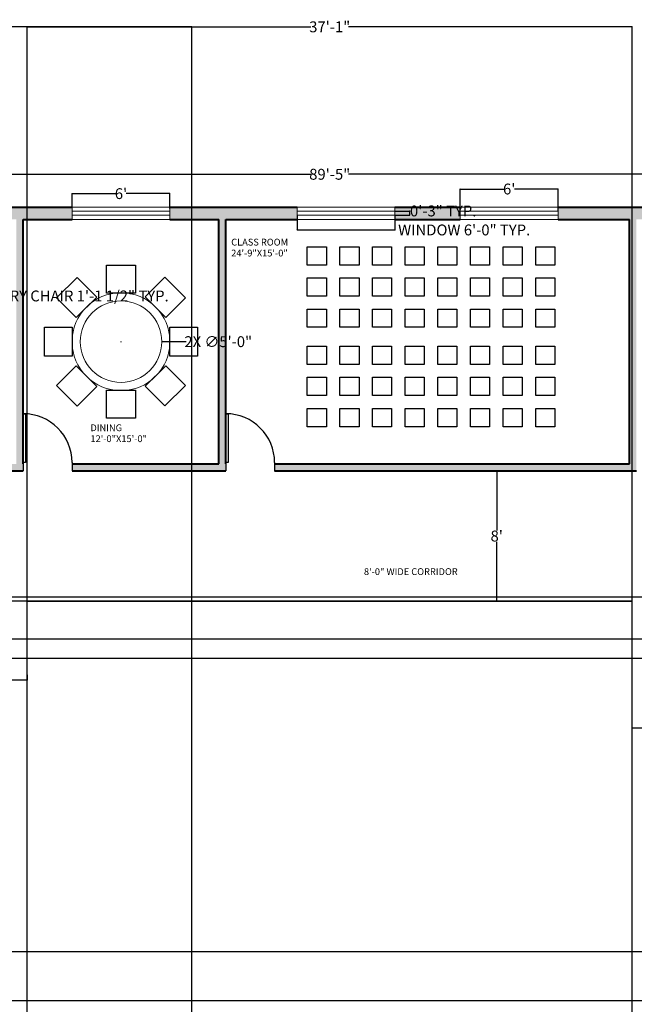
# Model space of a CAD drawing. Units: inches. Extents: x -405 to 940, y 226 to 2032.
# Tile 8 of 10: x 51 to 503, y 1301 to 2026. Entities that reach past the tile are written whole.
import ezdxf

# ---------------------------------------------------------------- set-up
doc = ezdxf.new("R2010")
doc.units = ezdxf.units.IN
doc.header["$MEASUREMENT"] = 0
doc.linetypes.add('ACAD_ISO02W100', pattern=[15, 12, -3])
for name, color, linetype, lineweight in [('A-ANNO-DIMS', 120, 'Continuous', 18), ('A-AREA-IDEN', 32, 'Continuous', 18), ('A-FLOR-EDGE', 3, 'Continuous', 25), ('A-FURN-SEAT', 5, 'Continuous', 18), ('A-GLAZ-HIDN', 1, 'ACAD_ISO02W100', 18), ('A-WALL-PATT', 8, 'Continuous', 13), ('door', 6, 'Continuous', 25), ('tables', 2, 'Continuous', 18), ('wall', 3, 'Continuous', 40), ('window', 1, 'Continuous', 18)]:
    doc.layers.add(name, color=color, linetype=linetype, lineweight=lineweight)
doc.layers.add('beches', color=5, linetype='Continuous')
doc.styles.get("Standard").update_dxf_attribs({"font": 'arial.ttf'})
doc.dimstyles.get("Standard").update_dxf_attribs({"dimtxt": 8, "dimasz": 0.18, "dimexe": 0.18, "dimexo": 0.0625, "dimgap": 0.09, "dimtad": 0, "dimtih": 1, "dimtoh": 1, "dimdec": 0, "dimzin": 0, "dimdsep": 46, "dimlunit": 3, "dimtxsty": 'Standard', "dimblk": 'OBLIQUE', "dimcen": 0.09, "dimadec": 0, "dimazin": 0, "dimtfac": 1, "dimtdec": 0, "dimtofl": 0, "dimtmove": 0, "dimatfit": 3, "dimfxl": 1, "dimtolj": 1, "dimtzin": 0, "dimarcsym": 0})

# ---------------------------------------------------------------- blocks, each defined once
blk = doc.blocks.new('*U4')
for p, q in [((0, 0), (0, -6)), ((36, 0), (36, -6))]:
    blk.add_line(p, q)
blk.add_lwpolyline([(0, 0), (0, 36), (1.75, 36), (1.75, 0)], close=True)
blk.add_arc((0, 0), 36, 0, 90)
blk = doc.blocks.new('*U33')
at = {"layer": 'beches'}
blk.add_lwpolyline([(6.71, -7.02), (-6.71, -7.02), (-6.71, 7.02), (6.71, 7.02)], close=True, dxfattribs=at)
blk = doc.blocks.new('*U34')
at = {"layer": 'A-FURN-SEAT', "transparency": 16777216}
for p in [(-45.84, 168), (-45.84, 168, 12), (-45.84, 168, 24), (-45.84, 168, 36), (-45.84, 168, 48), (-45.84, 168, 60), (-45.84, 168, 72), (-45.84, 168, 84), (-45.84, 168, 96), (-45.84, 168, 108), (-45.84, 168, 120), (-45.84, 168, 132), (-22.92, 168), (-22.92, 168, 12), (-22.92, 168, 24), (-22.92, 168, 36), (-22.92, 168, 48), (-22.92, 168, 60), (-22.92, 168, 72), (-22.92, 168, 84), (-22.92, 168, 96), (-22.92, 168, 108), (-22.92, 168, 120), (-22.92, 168, 132), (0, 168), (0, 168, 12), (0, 168, 24), (0, 168, 36), (0, 168, 48), (0, 168, 60), (0, 168, 72), (0, 168, 84), (0, 168, 96), (0, 168, 108), (0, 168, 120), (0, 168, 132), (-45.84, 144), (-45.84, 144, 12), (-45.84, 144, 24), (-45.84, 144, 36), (-45.84, 144, 48), (-45.84, 144, 60), (-45.84, 144, 72), (-45.84, 144, 84), (-45.84, 144, 96), (-45.84, 144, 108), (-45.84, 144, 120), (-45.84, 144, 132), (-22.92, 144), (-22.92, 144, 12), (-22.92, 144, 24), (-22.92, 144, 36), (-22.92, 144, 48), (-22.92, 144, 60), (-22.92, 144, 72), (-22.92, 144, 84), (-22.92, 144, 96), (-22.92, 144, 108), (-22.92, 144, 120), (-22.92, 144, 132), (0, 144), (0, 144, 12), (0, 144, 24), (0, 144, 36), (0, 144, 48), (0, 144, 60), (0, 144, 72), (0, 144, 84), (0, 144, 96), (0, 144, 108), (0, 144, 120), (0, 144, 132), (-45.84, 120), (-45.84, 120, 12), (-45.84, 120, 24), (-45.84, 120, 36), (-45.84, 120, 48), (-45.84, 120, 60), (-45.84, 120, 72), (-45.84, 120, 84), (-45.84, 120, 96), (-45.84, 120, 108), (-45.84, 120, 120), (-45.84, 120, 132), (-22.92, 120), (-22.92, 120, 12), (-22.92, 120, 24), (-22.92, 120, 36), (-22.92, 120, 48), (-22.92, 120, 60), (-22.92, 120, 72), (-22.92, 120, 84), (-22.92, 120, 96), (-22.92, 120, 108), (-22.92, 120, 120), (-22.92, 120, 132), (0, 120), (0, 120, 12), (0, 120, 24), (0, 120, 36), (0, 120, 48), (0, 120, 60), (0, 120, 72), (0, 120, 84), (0, 120, 96), (0, 120, 108), (0, 120, 120), (0, 120, 132), (-45.84, 96), (-45.84, 96, 12), (-45.84, 96, 24), (-45.84, 96, 36), (-45.84, 96, 48), (-45.84, 96, 60), (-45.84, 96, 72), (-45.84, 96, 84), (-45.84, 96, 96), (-45.84, 96, 108), (-45.84, 96, 120), (-45.84, 96, 132), (-22.92, 96), (-22.92, 96, 12), (-22.92, 96, 24), (-22.92, 96, 36), (-22.92, 96, 48), (-22.92, 96, 60), (-22.92, 96, 72), (-22.92, 96, 84), (-22.92, 96, 96), (-22.92, 96, 108), (-22.92, 96, 120), (-22.92, 96, 132), (0, 96), (0, 96, 12), (0, 96, 24), (0, 96, 36), (0, 96, 48), (0, 96, 60), (0, 96, 72), (0, 96, 84), (0, 96, 96), (0, 96, 108), (0, 96, 120), (0, 96, 132), (-45.84, 72), (-45.84, 72, 12), (-45.84, 72, 24), (-45.84, 72, 36), (-45.84, 72, 48), (-45.84, 72, 60), (-45.84, 72, 72), (-45.84, 72, 84), (-45.84, 72, 96), (-45.84, 72, 108), (-45.84, 72, 120), (-45.84, 72, 132), (-22.92, 72), (-22.92, 72, 12), (-22.92, 72, 24), (-22.92, 72, 36), (-22.92, 72, 48), (-22.92, 72, 60), (-22.92, 72, 72), (-22.92, 72, 84), (-22.92, 72, 96), (-22.92, 72, 108), (-22.92, 72, 120), (-22.92, 72, 132), (0, 72), (0, 72, 12), (0, 72, 24), (0, 72, 36), (0, 72, 48), (0, 72, 60), (0, 72, 72), (0, 72, 84), (0, 72, 96), (0, 72, 108), (0, 72, 120), (0, 72, 132), (-45.84, 48), (-45.84, 48, 12), (-45.84, 48, 24), (-45.84, 48, 36), (-45.84, 48, 48), (-45.84, 48, 60), (-45.84, 48, 72), (-45.84, 48, 84), (-45.84, 48, 96), (-45.84, 48, 108), (-45.84, 48, 120), (-45.84, 48, 132), (-22.92, 48), (-22.92, 48, 12), (-22.92, 48, 24), (-22.92, 48, 36), (-22.92, 48, 48), (-22.92, 48, 60), (-22.92, 48, 72), (-22.92, 48, 84), (-22.92, 48, 96), (-22.92, 48, 108), (-22.92, 48, 120), (-22.92, 48, 132), (0, 48), (0, 48, 12), (0, 48, 24), (0, 48, 36), (0, 48, 48), (0, 48, 60), (0, 48, 72), (0, 48, 84), (0, 48, 96), (0, 48, 108), (0, 48, 120), (0, 48, 132), (-45.84, 24), (-45.84, 24, 12), (-45.84, 24, 24), (-45.84, 24, 36), (-45.84, 24, 48), (-45.84, 24, 60), (-45.84, 24, 72), (-45.84, 24, 84), (-45.84, 24, 96), (-45.84, 24, 108), (-45.84, 24, 120), (-45.84, 24, 132), (-22.92, 24), (-22.92, 24, 12), (-22.92, 24, 24), (-22.92, 24, 36), (-22.92, 24, 48), (-22.92, 24, 60), (-22.92, 24, 72), (-22.92, 24, 84), (-22.92, 24, 96), (-22.92, 24, 108), (-22.92, 24, 120), (-22.92, 24, 132), (0, 24), (0, 24, 12), (0, 24, 24), (0, 24, 36), (0, 24, 48), (0, 24, 60), (0, 24, 72), (0, 24, 84), (0, 24, 96), (0, 24, 108), (0, 24, 120), (0, 24, 132), (-45.84, 0), (-45.84, 0, 12), (-45.84, 0, 24), (-45.84, 0, 36), (-45.84, 0, 48), (-45.84, 0, 60), (-45.84, 0, 72), (-45.84, 0, 84), (-45.84, 0, 96), (-45.84, 0, 108), (-45.84, 0, 120), (-45.84, 0, 132), (-22.92, 0), (-22.92, 0, 12), (-22.92, 0, 24), (-22.92, 0, 36), (-22.92, 0, 48), (-22.92, 0, 60), (-22.92, 0, 72), (-22.92, 0, 84), (-22.92, 0, 96), (-22.92, 0, 108), (-22.92, 0, 120), (-22.92, 0, 132), (0, 0), (0, 0, 12), (0, 0, 24), (0, 0, 36), (0, 0, 48), (0, 0, 60), (0, 0, 72), (0, 0, 84), (0, 0, 96), (0, 0, 108), (0, 0, 120), (0, 0, 132)]:
    blk.add_blockref('*U33', p, dxfattribs=at)
blk = doc.blocks.new('*U31')
at = {"layer": 'beches'}
blk.add_lwpolyline([(6.71, -7.02), (-6.71, -7.02), (-6.71, 7.02), (6.71, 7.02)], close=True, dxfattribs=at)
blk = doc.blocks.new('*U32')
at = {"layer": 'A-FURN-SEAT', "transparency": 16777216}
for p in [(-45.84, 168), (-45.84, 168, 12), (-45.84, 168, 24), (-45.84, 168, 36), (-45.84, 168, 48), (-45.84, 168, 60), (-45.84, 168, 72), (-45.84, 168, 84), (-45.84, 168, 96), (-45.84, 168, 108), (-45.84, 168, 120), (-45.84, 168, 132), (-22.92, 168), (-22.92, 168, 12), (-22.92, 168, 24), (-22.92, 168, 36), (-22.92, 168, 48), (-22.92, 168, 60), (-22.92, 168, 72), (-22.92, 168, 84), (-22.92, 168, 96), (-22.92, 168, 108), (-22.92, 168, 120), (-22.92, 168, 132), (0, 168), (0, 168, 12), (0, 168, 24), (0, 168, 36), (0, 168, 48), (0, 168, 60), (0, 168, 72), (0, 168, 84), (0, 168, 96), (0, 168, 108), (0, 168, 120), (0, 168, 132), (-45.84, 144), (-45.84, 144, 12), (-45.84, 144, 24), (-45.84, 144, 36), (-45.84, 144, 48), (-45.84, 144, 60), (-45.84, 144, 72), (-45.84, 144, 84), (-45.84, 144, 96), (-45.84, 144, 108), (-45.84, 144, 120), (-45.84, 144, 132), (-22.92, 144), (-22.92, 144, 12), (-22.92, 144, 24), (-22.92, 144, 36), (-22.92, 144, 48), (-22.92, 144, 60), (-22.92, 144, 72), (-22.92, 144, 84), (-22.92, 144, 96), (-22.92, 144, 108), (-22.92, 144, 120), (-22.92, 144, 132), (0, 144), (0, 144, 12), (0, 144, 24), (0, 144, 36), (0, 144, 48), (0, 144, 60), (0, 144, 72), (0, 144, 84), (0, 144, 96), (0, 144, 108), (0, 144, 120), (0, 144, 132), (-45.84, 120), (-45.84, 120, 12), (-45.84, 120, 24), (-45.84, 120, 36), (-45.84, 120, 48), (-45.84, 120, 60), (-45.84, 120, 72), (-45.84, 120, 84), (-45.84, 120, 96), (-45.84, 120, 108), (-45.84, 120, 120), (-45.84, 120, 132), (-22.92, 120), (-22.92, 120, 12), (-22.92, 120, 24), (-22.92, 120, 36), (-22.92, 120, 48), (-22.92, 120, 60), (-22.92, 120, 72), (-22.92, 120, 84), (-22.92, 120, 96), (-22.92, 120, 108), (-22.92, 120, 120), (-22.92, 120, 132), (0, 120), (0, 120, 12), (0, 120, 24), (0, 120, 36), (0, 120, 48), (0, 120, 60), (0, 120, 72), (0, 120, 84), (0, 120, 96), (0, 120, 108), (0, 120, 120), (0, 120, 132), (-45.84, 96), (-45.84, 96, 12), (-45.84, 96, 24), (-45.84, 96, 36), (-45.84, 96, 48), (-45.84, 96, 60), (-45.84, 96, 72), (-45.84, 96, 84), (-45.84, 96, 96), (-45.84, 96, 108), (-45.84, 96, 120), (-45.84, 96, 132), (-22.92, 96), (-22.92, 96, 12), (-22.92, 96, 24), (-22.92, 96, 36), (-22.92, 96, 48), (-22.92, 96, 60), (-22.92, 96, 72), (-22.92, 96, 84), (-22.92, 96, 96), (-22.92, 96, 108), (-22.92, 96, 120), (-22.92, 96, 132), (0, 96), (0, 96, 12), (0, 96, 24), (0, 96, 36), (0, 96, 48), (0, 96, 60), (0, 96, 72), (0, 96, 84), (0, 96, 96), (0, 96, 108), (0, 96, 120), (0, 96, 132), (-45.84, 72), (-45.84, 72, 12), (-45.84, 72, 24), (-45.84, 72, 36), (-45.84, 72, 48), (-45.84, 72, 60), (-45.84, 72, 72), (-45.84, 72, 84), (-45.84, 72, 96), (-45.84, 72, 108), (-45.84, 72, 120), (-45.84, 72, 132), (-22.92, 72), (-22.92, 72, 12), (-22.92, 72, 24), (-22.92, 72, 36), (-22.92, 72, 48), (-22.92, 72, 60), (-22.92, 72, 72), (-22.92, 72, 84), (-22.92, 72, 96), (-22.92, 72, 108), (-22.92, 72, 120), (-22.92, 72, 132), (0, 72), (0, 72, 12), (0, 72, 24), (0, 72, 36), (0, 72, 48), (0, 72, 60), (0, 72, 72), (0, 72, 84), (0, 72, 96), (0, 72, 108), (0, 72, 120), (0, 72, 132), (-45.84, 48), (-45.84, 48, 12), (-45.84, 48, 24), (-45.84, 48, 36), (-45.84, 48, 48), (-45.84, 48, 60), (-45.84, 48, 72), (-45.84, 48, 84), (-45.84, 48, 96), (-45.84, 48, 108), (-45.84, 48, 120), (-45.84, 48, 132), (-22.92, 48), (-22.92, 48, 12), (-22.92, 48, 24), (-22.92, 48, 36), (-22.92, 48, 48), (-22.92, 48, 60), (-22.92, 48, 72), (-22.92, 48, 84), (-22.92, 48, 96), (-22.92, 48, 108), (-22.92, 48, 120), (-22.92, 48, 132), (0, 48), (0, 48, 12), (0, 48, 24), (0, 48, 36), (0, 48, 48), (0, 48, 60), (0, 48, 72), (0, 48, 84), (0, 48, 96), (0, 48, 108), (0, 48, 120), (0, 48, 132), (-45.84, 24), (-45.84, 24, 12), (-45.84, 24, 24), (-45.84, 24, 36), (-45.84, 24, 48), (-45.84, 24, 60), (-45.84, 24, 72), (-45.84, 24, 84), (-45.84, 24, 96), (-45.84, 24, 108), (-45.84, 24, 120), (-45.84, 24, 132), (-22.92, 24), (-22.92, 24, 12), (-22.92, 24, 24), (-22.92, 24, 36), (-22.92, 24, 48), (-22.92, 24, 60), (-22.92, 24, 72), (-22.92, 24, 84), (-22.92, 24, 96), (-22.92, 24, 108), (-22.92, 24, 120), (-22.92, 24, 132), (0, 24), (0, 24, 12), (0, 24, 24), (0, 24, 36), (0, 24, 48), (0, 24, 60), (0, 24, 72), (0, 24, 84), (0, 24, 96), (0, 24, 108), (0, 24, 120), (0, 24, 132), (-45.84, 0), (-45.84, 0, 12), (-45.84, 0, 24), (-45.84, 0, 36), (-45.84, 0, 48), (-45.84, 0, 60), (-45.84, 0, 72), (-45.84, 0, 84), (-45.84, 0, 96), (-45.84, 0, 108), (-45.84, 0, 120), (-45.84, 0, 132), (-22.92, 0), (-22.92, 0, 12), (-22.92, 0, 24), (-22.92, 0, 36), (-22.92, 0, 48), (-22.92, 0, 60), (-22.92, 0, 72), (-22.92, 0, 84), (-22.92, 0, 96), (-22.92, 0, 108), (-22.92, 0, 120), (-22.92, 0, 132), (0, 0), (0, 0, 12), (0, 0, 24), (0, 0, 36), (0, 0, 48), (0, 0, 60), (0, 0, 72), (0, 0, 84), (0, 0, 96), (0, 0, 108), (0, 0, 120), (0, 0, 132)]:
    blk.add_blockref('*U31', p, dxfattribs=at)
blk = doc.blocks.new('*U35')
at = {"layer": 'beches'}
blk.add_lwpolyline([(-10.7, 10.22), (10.7, 10.22), (10.7, -10.22), (-10.7, -10.22)], close=True, dxfattribs=at)
blk = doc.blocks.new('*U36')
at = {"layer": 'A-FURN-SEAT', "transparency": 16777216}
blk.add_blockref('*U35', (125.75, 1834.83), dxfattribs=at)
for p, rotation in [((93.21, 1821.33), 45.00000000000002), ((158.29, 1821.37), 314.9999999999999), ((79.75, 1788.79), 90.00000000000003), ((171.79, 1788.83), 270), ((93.24, 1756.26), 135), ((158.32, 1756.29), 225), ((125.79, 1742.79), 180)]:
    blk.add_blockref('*U35', p, dxfattribs=dict(at, rotation=rotation))
blk = doc.blocks.new('_Oblique')
at = {"color": 0, "linetype": 'ByBlock', "lineweight": -2}
blk.add_line((-0.5, -0.5), (0.5, 0.5), dxfattribs=at)
blk = doc.blocks.new('*D40')
at = {"layer": 'A-ANNO-DIMS', "color": 0, "lineweight": -2, "transparency": 16777216}
for p, q in [((-39.23, 1543.59), (-39.23, 1539.64)), ((56.77, 1543.59), (56.77, 1539.64)), ((-39.23, 1539.82), (4.99, 1539.82)), ((56.77, 1539.82), (12.54, 1539.82))]:
    blk.add_line(p, q, dxfattribs=at)
at = {"layer": 'Defpoints', "color": 0, "transparency": 16777216}
for p in [(-39.23, 1543.65), (56.77, 1543.65), (56.77, 1539.82)]:
    blk.add_point(p, dxfattribs=at)
at = {"layer": 'A-ANNO-DIMS', "color": 0, "lineweight": -2, "transparency": 16777216, "xscale": 0.18, "yscale": 0.18, "zscale": 0.18, "rotation": 180}
blk.add_blockref('_Oblique', (-39.23, 1539.82), dxfattribs=at)
at = {"layer": 'A-ANNO-DIMS', "color": 0, "lineweight": -2, "transparency": 16777216, "xscale": 0.18, "yscale": 0.18, "zscale": 0.18}
blk.add_blockref('_Oblique', (56.77, 1539.82), dxfattribs=at)
at = {"layer": 'A-ANNO-DIMS', "color": 0, "transparency": 16777216, "insert": (8.77, 1539.82), "char_height": 8, "attachment_point": 5}
blk.add_mtext("\\A1;8'", dxfattribs=at)
blk = doc.blocks.new('*D41')
at = {"layer": 'A-ANNO-DIMS', "color": 0, "lineweight": -2, "transparency": 16777216}
for p, q in [((405.58, 1693.81), (401.92, 1693.81)), ((402.1, 1693.81), (402.1, 1649.98)), ((402.1, 1597.81), (402.1, 1641.64)), ((405.58, 1597.81), (401.92, 1597.81))]:
    blk.add_line(p, q, dxfattribs=at)
at = {"layer": 'Defpoints', "color": 0, "transparency": 16777216}
for p in [(405.64, 1693.81), (402.1, 1597.81), (405.64, 1597.81)]:
    blk.add_point(p, dxfattribs=at)
at = {"layer": 'A-ANNO-DIMS', "color": 0, "lineweight": -2, "transparency": 16777216, "xscale": 0.18, "yscale": 0.18, "zscale": 0.18}
for p, rotation in [((402.1, 1693.81), 90), ((402.1, 1597.81), 270)]:
    blk.add_blockref('_Oblique', p, dxfattribs=dict(at, rotation=rotation))
at = {"layer": 'A-ANNO-DIMS', "color": 0, "transparency": 16777216, "insert": (402.1, 1645.81), "char_height": 8, "attachment_point": 5}
blk.add_mtext("\\A1;8'", dxfattribs=at)
blk = doc.blocks.new('*D42')
at = {"layer": 'A-ANNO-DIMS', "color": 0, "lineweight": -2, "transparency": 16777216}
for p, q in [((501.77, 1498.93), (501.77, 1504.9)), ((501.77, 1504.72), (545.99, 1504.72)), ((597.77, 1504.72), (553.54, 1504.72)), ((597.77, 1498.93), (597.77, 1504.9))]:
    blk.add_line(p, q, dxfattribs=at)
at = {"layer": 'Defpoints', "color": 0, "transparency": 16777216}
for p in [(501.77, 1504.72), (501.77, 1498.87), (597.77, 1498.87)]:
    blk.add_point(p, dxfattribs=at)
at = {"layer": 'A-ANNO-DIMS', "color": 0, "lineweight": -2, "transparency": 16777216, "xscale": 0.18, "yscale": 0.18, "zscale": 0.18, "rotation": 180}
blk.add_blockref('_Oblique', (501.77, 1504.72), dxfattribs=at)
at = {"layer": 'A-ANNO-DIMS', "color": 0, "lineweight": -2, "transparency": 16777216, "xscale": 0.18, "yscale": 0.18, "zscale": 0.18}
blk.add_blockref('_Oblique', (597.77, 1504.72), dxfattribs=at)
at = {"layer": 'A-ANNO-DIMS', "color": 0, "transparency": 16777216, "insert": (549.77, 1504.72), "char_height": 8, "attachment_point": 5}
blk.add_mtext("\\A1;8'", dxfattribs=at)
blk = doc.blocks.new('*D43')
at = {"layer": 'A-ANNO-DIMS', "color": 0, "lineweight": -2, "transparency": 16777216}
for p, q in [((-257.23, 1887.87), (-257.23, 1912.15)), ((-257.23, 1911.97), (265.43, 1911.97)), ((815.77, 1911.97), (293.1, 1911.97)), ((815.77, 1887.87), (815.77, 1912.15))]:
    blk.add_line(p, q, dxfattribs=at)
at = {"layer": 'Defpoints', "color": 0, "transparency": 16777216}
for p in [(815.77, 1911.97), (-257.23, 1887.81), (815.77, 1887.81)]:
    blk.add_point(p, dxfattribs=at)
at = {"layer": 'A-ANNO-DIMS', "color": 0, "lineweight": -2, "transparency": 16777216, "xscale": 0.18, "yscale": 0.18, "zscale": 0.18, "rotation": 180}
blk.add_blockref('_Oblique', (-257.23, 1911.97), dxfattribs=at)
at = {"layer": 'A-ANNO-DIMS', "color": 0, "lineweight": -2, "transparency": 16777216, "xscale": 0.18, "yscale": 0.18, "zscale": 0.18}
blk.add_blockref('_Oblique', (815.77, 1911.97), dxfattribs=at)
at = {"layer": 'A-ANNO-DIMS', "color": 0, "transparency": 16777216, "insert": (279.27, 1911.97), "char_height": 8, "attachment_point": 5}
blk.add_mtext('\\A1;89\'-5"', dxfattribs=at)
blk = doc.blocks.new('*D63')
at = {"layer": 'A-ANNO-DIMS', "color": 0, "lineweight": -2, "transparency": 16777216}
for p, q in [((89.77, 1887.87), (89.77, 1897.91)), ((89.77, 1897.73), (121.98, 1897.73)), ((161.77, 1897.73), (129.56, 1897.73)), ((161.77, 1886.78), (161.77, 1897.91))]:
    blk.add_line(p, q, dxfattribs=at)
at = {"layer": 'Defpoints', "color": 0, "transparency": 16777216}
for p in [(161.77, 1897.73), (89.77, 1887.81), (161.77, 1886.72)]:
    blk.add_point(p, dxfattribs=at)
at = {"layer": 'A-ANNO-DIMS', "color": 0, "lineweight": -2, "transparency": 16777216, "xscale": 0.18, "yscale": 0.18, "zscale": 0.18, "rotation": 180}
blk.add_blockref('_Oblique', (89.77, 1897.73), dxfattribs=at)
at = {"layer": 'A-ANNO-DIMS', "color": 0, "lineweight": -2, "transparency": 16777216, "xscale": 0.18, "yscale": 0.18, "zscale": 0.18}
blk.add_blockref('_Oblique', (161.77, 1897.73), dxfattribs=at)
at = {"layer": 'A-ANNO-DIMS', "color": 0, "transparency": 16777216, "insert": (125.77, 1897.73), "char_height": 8, "attachment_point": 5}
blk.add_mtext("\\A1;6'", dxfattribs=at)
blk = doc.blocks.new('*D64')
at = {"layer": 'A-ANNO-DIMS', "color": 0, "lineweight": -2, "transparency": 16777216}
for p, q in [((375.27, 1884.87), (375.27, 1901.31)), ((375.27, 1901.13), (407.48, 1901.13)), ((447.27, 1901.13), (415.06, 1901.13)), ((447.27, 1884.87), (447.27, 1901.31))]:
    blk.add_line(p, q, dxfattribs=at)
at = {"layer": 'Defpoints', "color": 0, "transparency": 16777216}
for p in [(447.27, 1901.13), (375.27, 1884.81), (447.27, 1884.81)]:
    blk.add_point(p, dxfattribs=at)
at = {"layer": 'A-ANNO-DIMS', "color": 0, "lineweight": -2, "transparency": 16777216, "xscale": 0.18, "yscale": 0.18, "zscale": 0.18, "rotation": 180}
blk.add_blockref('_Oblique', (375.27, 1901.13), dxfattribs=at)
at = {"layer": 'A-ANNO-DIMS', "color": 0, "lineweight": -2, "transparency": 16777216, "xscale": 0.18, "yscale": 0.18, "zscale": 0.18}
blk.add_blockref('_Oblique', (447.27, 1901.13), dxfattribs=at)
at = {"layer": 'A-ANNO-DIMS', "color": 0, "transparency": 16777216, "insert": (411.27, 1901.13), "char_height": 8, "attachment_point": 5}
blk.add_mtext("\\A1;6'", dxfattribs=at)
blk = doc.blocks.new('TABLE-ROUND-72IN')
for radius in [36, 30]:
    blk.add_circle((36, 36), radius)
blk = doc.blocks.new('WIN-PANE-72IN')
for p, q in [((0, 3), (72, 3)), ((0, 0), (72, 0))]:
    blk.add_line(p, q)
blk = doc.blocks.new('*D83')
at = {"layer": 'A-ANNO-DIMS', "color": 0, "lineweight": -2, "transparency": 16777216}
for p, q in [((255.27, 1881.75), (255.27, 1870.83)), ((327.27, 1881.75), (327.27, 1870.83)), ((255.27, 1871.01), (327.27, 1871.01)), ((327.27, 1871.01), (327.45, 1871.01))]:
    blk.add_line(p, q, dxfattribs=at)
at = {"layer": 'Defpoints', "color": 0, "transparency": 16777216}
for p in [(255.27, 1881.81), (327.27, 1881.81), (327.27, 1871.01)]:
    blk.add_point(p, dxfattribs=at)
at = {"layer": 'A-ANNO-DIMS', "color": 0, "lineweight": -2, "transparency": 16777216, "xscale": 0.18, "yscale": 0.18, "zscale": 0.18, "rotation": 180}
blk.add_blockref('_Oblique', (255.27, 1871.01), dxfattribs=at)
at = {"layer": 'A-ANNO-DIMS', "color": 0, "lineweight": -2, "transparency": 16777216, "xscale": 0.18, "yscale": 0.18, "zscale": 0.18}
blk.add_blockref('_Oblique', (327.27, 1871.01), dxfattribs=at)
at = {"layer": 'A-ANNO-DIMS', "color": 0, "transparency": 16777216, "insert": (378.16, 1871.01), "char_height": 8, "attachment_point": 5}
blk.add_mtext('\\A1;WINDOW 6\'-0" TYP.', dxfattribs=at)
blk = doc.blocks.new('*D84')
at = {"layer": 'A-ANNO-DIMS', "color": 0, "lineweight": -2, "transparency": 16777216}
for p, q in [((327.33, 1884.81), (338.25, 1884.81)), ((338.07, 1884.81), (338.07, 1884.99)), ((338.07, 1884.99), (338.25, 1884.99)), ((338.07, 1881.81), (338.07, 1884.81)), ((327.33, 1881.81), (338.25, 1881.81))]:
    blk.add_line(p, q, dxfattribs=at)
at = {"layer": 'Defpoints', "color": 0, "transparency": 16777216}
for p in [(327.27, 1884.81), (338.07, 1884.81), (327.27, 1881.81)]:
    blk.add_point(p, dxfattribs=at)
at = {"layer": 'A-ANNO-DIMS', "color": 0, "lineweight": -2, "transparency": 16777216, "xscale": 0.18, "yscale": 0.18, "zscale": 0.18}
for p, rotation in [((338.07, 1884.81), 90), ((338.07, 1881.81), 270)]:
    blk.add_blockref('_Oblique', p, dxfattribs=dict(at, rotation=rotation))
at = {"layer": 'A-ANNO-DIMS', "color": 0, "transparency": 16777216, "insert": (362.72, 1884.99), "char_height": 8, "attachment_point": 5}
blk.add_mtext('\\A1;0\'-3" TYP.', dxfattribs=at)
blk = doc.blocks.new('*D91')
at = {"layer": 'A-ANNO-DIMS', "color": 0, "lineweight": -2, "transparency": 16777216}
for p, q in [((-2.26, 1824.45), (-2.26, 1822.27)), ((-2.26, 1822.45), (11.46, 1822.45)), ((11.46, 1824.45), (11.46, 1822.27)), ((11.46, 1822.45), (11.64, 1822.45))]:
    blk.add_line(p, q, dxfattribs=at)
at = {"layer": 'Defpoints', "color": 0, "transparency": 16777216}
for p in [(-2.26, 1824.51), (11.46, 1824.51), (11.46, 1822.45)]:
    blk.add_point(p, dxfattribs=at)
at = {"layer": 'A-ANNO-DIMS', "color": 0, "lineweight": -2, "transparency": 16777216, "xscale": 0.18, "yscale": 0.18, "zscale": 0.18, "rotation": 180}
blk.add_blockref('_Oblique', (-2.26, 1822.45), dxfattribs=at)
at = {"layer": 'A-ANNO-DIMS', "color": 0, "lineweight": -2, "transparency": 16777216, "xscale": 0.18, "yscale": 0.18, "zscale": 0.18}
blk.add_blockref('_Oblique', (11.46, 1822.45), dxfattribs=at)
at = {"layer": 'A-ANNO-DIMS', "color": 0, "transparency": 16777216, "insert": (88.39, 1822.45), "char_height": 8, "attachment_point": 5}
blk.add_mtext('\\A1;PANTRY CHAIR 1\'-1 1/2" TYP.', dxfattribs=at)
blk = doc.blocks.new('*D100')
at = {"layer": 'A-ANNO-DIMS', "color": 0, "lineweight": -2, "transparency": 16777216}
for p, q in [((626.71, 1569.84), (-390.06, 1569.84)), ((-389.88, 1569.84), (-389.88, 1566.93)), ((-389.88, 1555.81), (-389.88, 1558.72)), ((626.71, 1555.81), (-390.06, 1555.81))]:
    blk.add_line(p, q, dxfattribs=at)
at = {"layer": 'Defpoints', "color": 0, "transparency": 16777216}
for p in [(626.77, 1569.84), (-389.88, 1555.81), (626.77, 1555.81)]:
    blk.add_point(p, dxfattribs=at)
at = {"layer": 'A-ANNO-DIMS', "color": 0, "lineweight": -2, "transparency": 16777216, "xscale": 0.18, "yscale": 0.18, "zscale": 0.18}
for p, rotation in [((-389.88, 1569.84), 90), ((-389.88, 1555.81), 270)]:
    blk.add_blockref('_Oblique', p, dxfattribs=dict(at, rotation=rotation))
at = {"layer": 'A-ANNO-DIMS', "color": 0, "transparency": 16777216, "insert": (-389.88, 1562.83), "char_height": 8, "attachment_point": 5}
blk.add_mtext('\\A1;1\'-2"', dxfattribs=at)
blk = doc.blocks.new('*D105')
at = {"layer": 'A-ANNO-DIMS', "color": 0, "lineweight": -2, "transparency": 16777216}
for p, q in [((602.71, 1600.81), (-390.06, 1600.81)), ((-389.88, 1600.81), (-389.88, 1589.43)), ((-389.88, 1569.84), (-389.88, 1581.22)), ((626.71, 1569.84), (-390.06, 1569.84))]:
    blk.add_line(p, q, dxfattribs=at)
at = {"layer": 'Defpoints', "color": 0, "transparency": 16777216}
for p in [(602.77, 1600.81), (-389.88, 1569.84), (626.77, 1569.84)]:
    blk.add_point(p, dxfattribs=at)
at = {"layer": 'A-ANNO-DIMS', "color": 0, "lineweight": -2, "transparency": 16777216, "xscale": 0.18, "yscale": 0.18, "zscale": 0.18}
for p, rotation in [((-389.88, 1600.81), 90), ((-389.88, 1569.84), 270)]:
    blk.add_blockref('_Oblique', p, dxfattribs=dict(at, rotation=rotation))
at = {"layer": 'A-ANNO-DIMS', "color": 0, "transparency": 16777216, "insert": (-389.88, 1585.33), "char_height": 8, "attachment_point": 5}
blk.add_mtext('\\A1;2\'-7"', dxfattribs=at)
blk = doc.blocks.new('*D106')
at = {"layer": 'A-ANNO-DIMS', "color": 0, "lineweight": -2, "transparency": 16777216}
for p, q in [((56.77, 851.87), (56.77, 2020.64)), ((56.77, 2020.46), (265.44, 2020.46)), ((501.77, 2020.46), (293.1, 2020.46)), ((501.77, 851.87), (501.77, 2020.64))]:
    blk.add_line(p, q, dxfattribs=at)
at = {"layer": 'Defpoints', "color": 0, "transparency": 16777216}
for p in [(501.77, 2020.46), (56.77, 851.81), (501.77, 851.81)]:
    blk.add_point(p, dxfattribs=at)
at = {"layer": 'A-ANNO-DIMS', "color": 0, "lineweight": -2, "transparency": 16777216, "xscale": 0.18, "yscale": 0.18, "zscale": 0.18, "rotation": 180}
blk.add_blockref('_Oblique', (56.77, 2020.46), dxfattribs=at)
at = {"layer": 'A-ANNO-DIMS', "color": 0, "lineweight": -2, "transparency": 16777216, "xscale": 0.18, "yscale": 0.18, "zscale": 0.18}
blk.add_blockref('_Oblique', (501.77, 2020.46), dxfattribs=at)
at = {"layer": 'A-ANNO-DIMS', "color": 0, "transparency": 16777216, "insert": (279.27, 2020.46), "char_height": 8, "attachment_point": 5}
blk.add_mtext('\\A1;37\'-1"', dxfattribs=at)
blk = doc.blocks.new('*D107')
at = {"layer": 'A-ANNO-DIMS', "color": 0, "lineweight": -2, "transparency": 16777216}
for p, q in [((501.71, 1597.81), (-390.06, 1597.81)), ((-389.88, 1597.81), (-389.88, 1228.98)), ((-389.88, 851.81), (-389.88, 1220.64)), ((501.71, 851.81), (-390.06, 851.81))]:
    blk.add_line(p, q, dxfattribs=at)
at = {"layer": 'Defpoints', "color": 0, "transparency": 16777216}
for p in [(-389.88, 1597.81), (501.77, 1597.81), (501.77, 851.81)]:
    blk.add_point(p, dxfattribs=at)
at = {"layer": 'A-ANNO-DIMS', "color": 0, "lineweight": -2, "transparency": 16777216, "xscale": 0.18, "yscale": 0.18, "zscale": 0.18}
for p, rotation in [((-389.88, 1597.81), 90), ((-389.88, 851.81), 270)]:
    blk.add_blockref('_Oblique', p, dxfattribs=dict(at, rotation=rotation))
at = {"layer": 'A-ANNO-DIMS', "color": 0, "transparency": 16777216, "insert": (-389.88, 1224.81), "char_height": 8, "attachment_point": 5}
blk.add_mtext('\\A1;62\'-2"', dxfattribs=at)
blk = doc.blocks.new('*D109')
at = {"layer": 'A-ANNO-DIMS', "color": 0, "lineweight": -2, "transparency": 16777216}
for p, q in [((-248.23, 750.87), (-248.23, 2020.64)), ((-248.23, 2020.46), (-49.06, 2020.46)), ((177.77, 2020.46), (-21.4, 2020.46)), ((177.77, 750.87), (177.77, 2020.64))]:
    blk.add_line(p, q, dxfattribs=at)
at = {"layer": 'Defpoints', "color": 0, "transparency": 16777216}
for p in [(177.77, 2020.46), (-248.23, 750.81), (177.77, 750.81)]:
    blk.add_point(p, dxfattribs=at)
at = {"layer": 'A-ANNO-DIMS', "color": 0, "lineweight": -2, "transparency": 16777216, "xscale": 0.18, "yscale": 0.18, "zscale": 0.18, "rotation": 180}
blk.add_blockref('_Oblique', (-248.23, 2020.46), dxfattribs=at)
at = {"layer": 'A-ANNO-DIMS', "color": 0, "lineweight": -2, "transparency": 16777216, "xscale": 0.18, "yscale": 0.18, "zscale": 0.18}
blk.add_blockref('_Oblique', (177.77, 2020.46), dxfattribs=at)
at = {"layer": 'A-ANNO-DIMS', "color": 0, "transparency": 16777216, "insert": (-35.23, 2020.46), "char_height": 8, "attachment_point": 5}
blk.add_mtext('\\A1;35\'-6"', dxfattribs=at)
blk = doc.blocks.new('*D114')
at = {"layer": 'A-ANNO-DIMS', "color": 0, "lineweight": -2, "transparency": 16777216}
for p, q in [((602.71, 1339.81), (-390.06, 1339.81)), ((-389.88, 1339.81), (-389.88, 1325.99)), ((-389.88, 1303.81), (-389.88, 1317.63)), ((602.71, 1303.81), (-390.06, 1303.81))]:
    blk.add_line(p, q, dxfattribs=at)
at = {"layer": 'Defpoints', "color": 0, "transparency": 16777216}
for p in [(602.77, 1339.81), (-389.88, 1303.81), (602.77, 1303.81)]:
    blk.add_point(p, dxfattribs=at)
at = {"layer": 'A-ANNO-DIMS', "color": 0, "lineweight": -2, "transparency": 16777216, "xscale": 0.18, "yscale": 0.18, "zscale": 0.18}
for p, rotation in [((-389.88, 1339.81), 90), ((-389.88, 1303.81), 270)]:
    blk.add_blockref('_Oblique', p, dxfattribs=dict(at, rotation=rotation))
at = {"layer": 'A-ANNO-DIMS', "color": 0, "transparency": 16777216, "insert": (-389.88, 1321.81), "char_height": 8, "attachment_point": 5}
blk.add_mtext('\\A1;3\'-0"', dxfattribs=at)
blk = doc.blocks.new('*D118')
at = {"layer": 'A-ANNO-DIMS', "color": 0, "lineweight": -2, "transparency": 16777216}
for p, q in [((125.68, 1788.81), (125.86, 1788.81)), ((125.77, 1788.72), (125.77, 1788.9)), ((173.77, 1788.81), (155.77, 1788.81))]:
    blk.add_line(p, q, dxfattribs=at)
at = {"layer": 'Defpoints', "color": 0, "transparency": 16777216}
for p in [(95.77, 1788.81), (155.77, 1788.81)]:
    blk.add_point(p, dxfattribs=at)
at = {"layer": 'A-ANNO-DIMS', "color": 0, "lineweight": -2, "transparency": 16777216, "xscale": 0.18, "yscale": 0.18, "zscale": 0.18, "rotation": 179.9996944225092}
blk.add_blockref('_Oblique', (155.77, 1788.81), dxfattribs=at)
at = {"layer": 'A-ANNO-DIMS', "color": 0, "transparency": 16777216, "insert": (197.29, 1788.81), "char_height": 8, "attachment_point": 5}
blk.add_mtext('\\A1;2X ∅5\'-0"', dxfattribs=at)

msp = doc.modelspace()

# ---------------------------------------------------------------- hatches: boundary and pattern name
at = {"layer": 'A-WALL-PATT'}
h = msp.add_hatch(dxfattribs=at)
h.set_pattern_fill('AR-HBONE', color=256)
h.set_pattern_definition([(45, (599.8442, 904.9158), (0, 5.656854), [12, -4]), (135, (602.6726, 907.744), (4e-16, 5.656854), [12, -4])])
h.paths.add_polyline_path([(-248.23, 1045.81), (-257.23, 1045.81), (-257.23, 964.81), (-248.23, 964.81)], flags=17)
h.paths.add_polyline_path([(-248.23, 851.81), (-39.23, 851.81), (-39.23, 856.81), (-44.23, 856.81), (-248.23, 856.81), (-248.23, 892.81), (-257.23, 892.81), (-257.23, 839.81), (-248.23, 839.81)])
h.paths.add_polyline_path([(-248.23, 750.81), (124.74, 750.81), (124.74, 751.73), (124.74, 755.81), (-248.23, 755.81), (-248.23, 767.81), (-257.23, 767.81), (-257.23, 726.81), (-248.23, 726.81)])
h.paths.add_polyline_path([(-248.23, 654.81), (-257.23, 654.81), (-257.23, 630.81), (-248.23, 630.81)])
h.paths.add_polyline_path([(-180.23, 534.81), (-248.23, 534.81), (-248.23, 558.81), (-257.23, 558.81), (-257.23, 525.81), (-180.23, 525.81)])
h.paths.add_polyline_path([(-69.23, 534.81), (-108.23, 534.81), (-108.23, 525.81), (-69.23, 525.81)])
h.paths.add_polyline_path([(35.77, 534.81), (2.77, 534.81), (2.77, 525.81), (35.77, 525.81)])
h.paths.add_polyline_path([(182.77, 755.81), (160.74, 755.81), (160.74, 750.81), (177.77, 750.81), (177.77, 534.81), (107.77, 534.81), (107.77, 525.81), (182.77, 525.81)])
h.paths.add_polyline_path([(-39.23, 1609.81), (-44.23, 1609.81), (-44.23, 1604.81), (-44.23, 1460.81), (-135.23, 1460.81), (-135.23, 1465.73), (-140.23, 1465.73), (-140.23, 1460.81), (-248.23, 1460.81), (-248.23, 1471.31), (-257.23, 1471.31), (-257.23, 1419.81), (-248.23, 1419.81), (-248.23, 1455.81), (-44.23, 1455.81), (-44.23, 1194.81), (-39.23, 1194.81)])
h.paths.add_polyline_path([(-248.23, 1520.81), (-257.23, 1520.81), (-257.23, 1495.31), (-248.23, 1495.31), (-248.23, 1505.81), (-140.23, 1505.81), (-140.23, 1495.73), (-135.23, 1495.73), (-135.23, 1516.79), (-140.23, 1516.79), (-140.23, 1510.81), (-248.23, 1510.81)], flags=17)
h.paths.add_polyline_path([(-248.23, 1570.31), (-257.23, 1570.31), (-257.23, 1544.81), (-248.23, 1544.81), (-248.23, 1554.81), (-140.23, 1554.81), (-140.23, 1546.79), (-135.23, 1546.79), (-135.23, 1565.08), (-140.23, 1565.08), (-140.23, 1559.81), (-248.23, 1559.81)], flags=17)
h.paths.add_polyline_path([(-248.23, 1615.81), (-257.23, 1615.81), (-257.23, 1594.31), (-248.23, 1594.31), (-248.23, 1604.81), (-140.23, 1604.81), (-140.23, 1595.08), (-135.23, 1595.08), (-135.23, 1604.81), (-80.23, 1604.81), (-80.23, 1609.81), (-248.23, 1609.81)])
h.paths.add_polyline_path([(-248.23, 1783.81), (-235.46, 1783.81), (-235.46, 1788.81), (-248.23, 1788.81), (-248.23, 1878.81), (-237.73, 1878.81), (-237.73, 1887.81), (-257.23, 1887.81), (-257.23, 1687.81), (-248.23, 1687.81), (-248.23, 1693.81), (-136.23, 1693.81), (-136.23, 1698.81), (-248.23, 1698.81)])
h.paths.add_polyline_path([(-188.23, 1887.81), (-213.73, 1887.81), (-213.73, 1878.81), (-203.23, 1878.81), (-203.23, 1788.81), (-205.46, 1788.81), (-205.46, 1783.81), (-186.39, 1783.81), (-186.39, 1788.81), (-198.23, 1788.81), (-198.23, 1878.81), (-188.23, 1878.81)])
h.paths.add_polyline_path([(-139.23, 1887.81), (-164.23, 1887.81), (-164.23, 1878.81), (-154.23, 1878.81), (-154.23, 1788.81), (-156.39, 1788.81), (-156.39, 1783.81), (-138.25, 1783.81), (-138.25, 1788.81), (-149.23, 1788.81), (-149.23, 1878.81), (-139.23, 1878.81)])
h.paths.add_polyline_path([(-89.23, 1887.81), (-115.23, 1887.81), (-115.23, 1878.81), (-105.23, 1878.81), (-105.23, 1788.81), (-108.25, 1788.81), (-108.25, 1783.81), (-86.45, 1783.81), (-86.45, 1788.81), (-100.23, 1788.81), (-100.23, 1878.81), (-89.23, 1878.81)])
h.paths.add_polyline_path([(-36.23, 1887.81), (-65.23, 1887.81), (-65.23, 1878.81), (-54.23, 1878.81), (-54.23, 1788.81), (-56.45, 1788.81), (-56.45, 1783.81), (-54.23, 1783.81), (-54.23, 1698.81), (-100.23, 1698.81), (-100.23, 1693.81), (-49.23, 1693.81), (-49.23, 1698.81), (-49.23, 1878.81), (-36.23, 1878.81)])
h.paths.add_polyline_path([(89.77, 1887.81), (35.77, 1887.81), (35.77, 1878.81), (48.77, 1878.81), (48.77, 1698.81), (-13.23, 1698.81), (-13.23, 1693.81), (53.77, 1693.81), (53.77, 1698.81), (53.77, 1878.81), (89.77, 1878.81)])
h.paths.add_polyline_path([(255.27, 1887.81), (161.77, 1887.81), (161.77, 1878.81), (197.77, 1878.81), (197.77, 1698.81), (89.77, 1698.81), (89.77, 1693.81), (202.77, 1693.81), (202.77, 1698.81), (202.77, 1878.81), (255.27, 1878.81)])
h.paths.add_polyline_path([(375.27, 1887.81), (327.27, 1887.81), (327.27, 1878.81), (375.27, 1878.81)], flags=17)
h.paths.add_polyline_path([(815.77, 1887.81), (447.27, 1887.81), (447.27, 1878.81), (499.77, 1878.81), (499.77, 1698.81), (238.77, 1698.81), (238.77, 1693.81), (504.77, 1693.81), (504.77, 1878.81), (633.77, 1878.81), (633.77, 1646.81), (597.77, 1646.81), (597.77, 1641.81), (602.77, 1641.81), (638.77, 1641.81), (638.77, 1878.81), (806.77, 1878.81), (806.77, 1838.31), (815.77, 1838.31)])
h.paths.add_polyline_path([(815.77, 1766.31), (806.77, 1766.31), (806.77, 1718.31), (815.77, 1718.31)], flags=17)
h.paths.add_polyline_path([(815.77, 1356.31), (806.77, 1356.31), (806.77, 1303.81), (602.77, 1303.81), (597.77, 1303.81), (597.77, 1037.81), (602.77, 1037.81), (602.77, 1298.81), (806.77, 1298.81), (806.77, 1246.31), (815.77, 1246.31)])
h.paths.add_polyline_path([(815.77, 1174.31), (806.77, 1174.31), (806.77, 1126.31), (815.77, 1126.31)], flags=17)
h.paths.add_polyline_path([(815.77, 1054.31), (806.77, 1054.31), (806.77, 1001.81), (796.08, 1001.81), (796.08, 1001.75), (780.86, 1001.75), (602.77, 1001.81), (597.77, 1001.81), (597.77, 892.81), (602.77, 892.81), (602.77, 996.81), (806.77, 996.81), (806.77, 962.81), (815.77, 962.81)])
h.paths.add_polyline_path([(403.77, 534.81), (379.77, 534.81), (379.77, 525.81), (403.77, 525.81)])
h.paths.add_polyline_path([(-39.23, 1158.81), (-44.23, 1158.81), (-248.23, 1158.81), (-248.23, 1194.81), (-257.23, 1194.81), (-257.23, 1117.81), (-248.23, 1117.81), (-248.23, 1153.81), (-44.23, 1153.81), (-44.23, 892.81), (-39.23, 892.81)])
h.paths.add_polyline_path([(-248.23, 1347.81), (-257.23, 1347.81), (-257.23, 1275.81), (-248.23, 1275.81)], flags=17)
h.paths.add_polyline_path([(815.77, 1476.31), (806.77, 1476.31), (806.77, 1428.31), (815.77, 1428.31)], flags=17)
h.paths.add_polyline_path([(815.77, 1646.31), (806.77, 1646.31), (806.77, 1638.65), (806.77, 1605.81), (597.77, 1605.81), (597.77, 1339.81), (602.77, 1339.81), (602.77, 1600.81), (806.77, 1600.81), (806.77, 1548.31), (815.77, 1548.31)])

# ---------------------------------------------------------------- linework, layer by layer
at = {"layer": 'A-FLOR-EDGE'}
for p, q in [((56.77, 1597.81), (501.77, 1597.81)), ((56.77, 851.81), (56.77, 1597.81)), ((501.77, 851.81), (501.77, 1597.81))]:
    msp.add_line(p, q, dxfattribs=at)
at = {"layer": 'A-GLAZ-HIDN'}
for p, q in [((89.77, 1878.81), (89.77, 1887.81)), ((161.77, 1878.81), (161.77, 1887.81)), ((255.27, 1878.81), (255.27, 1887.81)), ((327.27, 1878.81), (327.27, 1887.81)), ((375.27, 1878.81), (375.27, 1887.81)), ((447.27, 1878.81), (447.27, 1887.81))]:
    msp.add_line(p, q, dxfattribs=at)
at = {"layer": 'door'}
for p, q in [((53.77, 1698.81), (53.77, 1693.81)), ((89.77, 1698.81), (89.77, 1693.81)), ((202.77, 1698.81), (202.77, 1693.81)), ((238.77, 1698.81), (238.77, 1693.81))]:
    msp.add_line(p, q, dxfattribs=at)
at = {"layer": 'wall'}
for p, q in [((35.77, 1887.81), (89.77, 1887.81)), ((161.77, 1887.81), (255.27, 1887.81)), ((327.27, 1887.81), (375.27, 1887.81)), ((447.27, 1887.81), (815.77, 1887.81)), ((53.77, 1698.81), (53.77, 1878.81)), ((53.77, 1878.81), (89.77, 1878.81)), ((161.77, 1878.81), (197.77, 1878.81)), ((197.77, 1698.81), (197.77, 1878.81)), ((202.77, 1698.81), (202.77, 1878.81)), ((202.77, 1878.81), (255.27, 1878.81)), ((327.27, 1878.81), (375.27, 1878.81)), ((447.27, 1878.81), (499.77, 1878.81)), ((499.77, 1698.81), (499.77, 1878.81)), ((89.77, 1698.81), (197.77, 1698.81)), ((238.77, 1698.81), (499.77, 1698.81)), ((-13.23, 1693.81), (53.77, 1693.81)), ((89.77, 1693.81), (202.77, 1693.81)), ((238.77, 1693.81), (504.77, 1693.81))]:
    msp.add_line(p, q, dxfattribs=at)
at = {"layer": 'window'}
for p, q in [((89.77, 1887.81), (161.77, 1887.81)), ((255.27, 1887.81), (327.27, 1887.81)), ((375.27, 1887.81), (447.27, 1887.81)), ((375.27, 1884.81), (447.27, 1884.81)), ((89.77, 1878.81), (161.77, 1878.81)), ((255.27, 1878.81), (327.27, 1878.81)), ((375.27, 1881.81), (447.27, 1881.81)), ((375.27, 1878.81), (447.27, 1878.81))]:
    msp.add_line(p, q, dxfattribs=at)

# ---------------------------------------------------------------- block references
at = {"layer": 'A-FURN-SEAT', "rotation": 270}
for name, p in [('*U32', (269.79, 1806.07)), ('*U34', (269.79, 1732.95))]:
    msp.add_blockref(name, p, dxfattribs=at)
at = {"layer": 'A-FURN-SEAT'}
msp.add_blockref('*U36', (0, 0), dxfattribs=at)
at = {"layer": 'door'}
for p in [(53.77, 1699.81), (202.77, 1699.81)]:
    msp.add_blockref('*U4', p, dxfattribs=at)
at = {"layer": 'tables'}
msp.add_blockref('TABLE-ROUND-72IN', (89.77, 1752.81), dxfattribs=at)
at = {"layer": 'window'}
for p in [(89.77, 1881.81), (255.27, 1881.81)]:
    msp.add_blockref('WIN-PANE-72IN', p, dxfattribs=at)

# ---------------------------------------------------------------- texts
at = {"layer": 'A-AREA-IDEN'}
for s, p in [('CLASS ROOM ', (206.81, 1859.54)), ('24\'-9"X15\'-0"', (206.81, 1851.51)), ('DINING ', (103.26, 1722.96)), ('12\'-0"X15\'-0"', (103.26, 1714.92)), ('8\'-0" WIDE CORRIDOR ', (304.42, 1617.11))]:
    msp.add_text(s, height=5, dxfattribs=at).set_placement(p)

# ---------------------------------------------------------------- dimensions: what is measured, and where the dimension line sits
at = {"layer": 'A-ANNO-DIMS'}
for base, p1, p2, override, picture, middle in [((177.77, 2020.46), (-248.23, 750.81), (177.77, 750.81), {"dimdec": 1, "dimlfac": 1, "dimrnd": 0, "dimzin": 1, "dimdsep": 46, "dimlunit": 4, "dimfrac": 2}, '*D109', (-35.23, 2020.46)), ((501.77, 2020.46), (56.77, 851.81), (501.77, 851.81), {"dimdec": 1, "dimlfac": 1, "dimrnd": 0, "dimzin": 1, "dimdsep": 46, "dimlunit": 4, "dimfrac": 2}, '*D106', (279.27, 2020.46)), ((815.77, 1911.97), (-257.23, 1887.81), (815.77, 1887.81), {"dimclrd": 0, "dimclre": 0, "dimclrt": 0}, '*D43', (279.27, 1911.97)), ((447.27, 1901.13), (375.27, 1884.81), (447.27, 1884.81), {"dimclrd": 0, "dimclre": 0, "dimclrt": 0}, '*D64', (411.27, 1901.13)), ((161.77, 1897.73), (89.77, 1887.81), (161.77, 1886.72), {"dimclrd": 0, "dimclre": 0, "dimclrt": 0}, '*D63', (125.77, 1897.73)), ((56.77, 1539.82), (-39.23, 1543.65), (56.77, 1543.65), {"dimclrd": 0, "dimclre": 0, "dimclrt": 0}, '*D40', (8.77, 1539.82)), ((501.77, 1504.72), (597.77, 1498.87), (501.77, 1498.87), {"dimclrd": 0, "dimclre": 0, "dimclrt": 0}, '*D42', (549.77, 1504.72))]:
    dim = msp.add_linear_dim(base=base, p1=p1, p2=p2, dimstyle='Standard', override=override, dxfattribs=at)
    dim.commit()
    dim.dimension.update_dxf_attribs({"geometry": picture, "text_midpoint": middle})
dim = msp.add_linear_dim(base=(338.07, 1884.81), p1=(327.27, 1881.81), p2=(327.27, 1884.81), angle=90, text='<> TYP.', dimstyle='Standard', override={"dimdec": 1, "dimlfac": 1, "dimrnd": 0, "dimzin": 1, "dimdsep": 46, "dimlunit": 4, "dimfrac": 2}, dxfattribs=at)
dim.commit()
dim.dimension.update_dxf_attribs({"geometry": '*D84', "text_midpoint": (362.72, 1884.99)})
for base, p1, p2, text, picture, middle in [((327.27, 1871.01), (255.27, 1881.81), (327.27, 1881.81), 'WINDOW <> TYP.', '*D83', (378.16, 1871.01)), ((11.46, 1822.45), (-2.26, 1824.51), (11.46, 1824.51), 'PANTRY CHAIR <> TYP.', '*D91', (88.39, 1822.45))]:
    dim = msp.add_linear_dim(base=base, p1=p1, p2=p2, text=text, dimstyle='Standard', override={"dimdec": 1, "dimlfac": 1, "dimrnd": 0, "dimzin": 1, "dimdsep": 46, "dimlunit": 4, "dimfrac": 2}, dxfattribs=at)
    dim.commit()
    dim.dimension.update_dxf_attribs({"geometry": picture, "text_midpoint": middle})
dim = msp.add_diameter_dim_2p(p1=(95.77, 1788.81), p2=(155.77, 1788.81), text='2X <>', dimstyle='Standard', override={"dimdec": 1, "dimlfac": 1, "dimrnd": 0, "dimzin": 1, "dimdsep": 46, "dimlunit": 4, "dimfrac": 2}, dxfattribs=at)
dim.commit()
dim.dimension.update_dxf_attribs({"geometry": '*D118', "text_midpoint": (173.77, 1788.81), "dimtype": 163})
for base, p1, p2, override, picture, middle in [((402.1, 1597.81), (405.64, 1693.81), (405.64, 1597.81), {"dimclrd": 0, "dimclre": 0, "dimclrt": 0}, '*D41', (402.1, 1645.81)), ((-389.88, 1597.81), (501.77, 851.81), (501.77, 1597.81), {"dimdec": 1, "dimlfac": 1, "dimrnd": 0, "dimzin": 1, "dimdsep": 46, "dimlunit": 4, "dimfrac": 2}, '*D107', (-389.88, 1224.81)), ((-389.88, 1569.84), (602.77, 1600.81), (626.77, 1569.84), {"dimdec": 1, "dimlfac": 1, "dimrnd": 0, "dimzin": 1, "dimdsep": 46, "dimlunit": 4, "dimfrac": 2}, '*D105', (-389.88, 1585.33)), ((-389.88, 1555.81), (626.77, 1569.84), (626.77, 1555.81), {"dimdec": 1, "dimlfac": 1, "dimrnd": 0, "dimzin": 1, "dimdsep": 46, "dimlunit": 4, "dimfrac": 2}, '*D100', (-389.88, 1562.83)), ((-389.88, 1303.81), (602.77, 1339.81), (602.77, 1303.81), {"dimdec": 1, "dimlfac": 1, "dimrnd": 0, "dimzin": 1, "dimdsep": 46, "dimlunit": 4, "dimfrac": 2}, '*D114', (-389.88, 1321.81))]:
    dim = msp.add_linear_dim(base=base, p1=p1, p2=p2, angle=90, dimstyle='Standard', override=override, dxfattribs=at)
    dim.commit()
    dim.dimension.update_dxf_attribs({"geometry": picture, "text_midpoint": middle})

doc.saveas('drawing.dxf')
